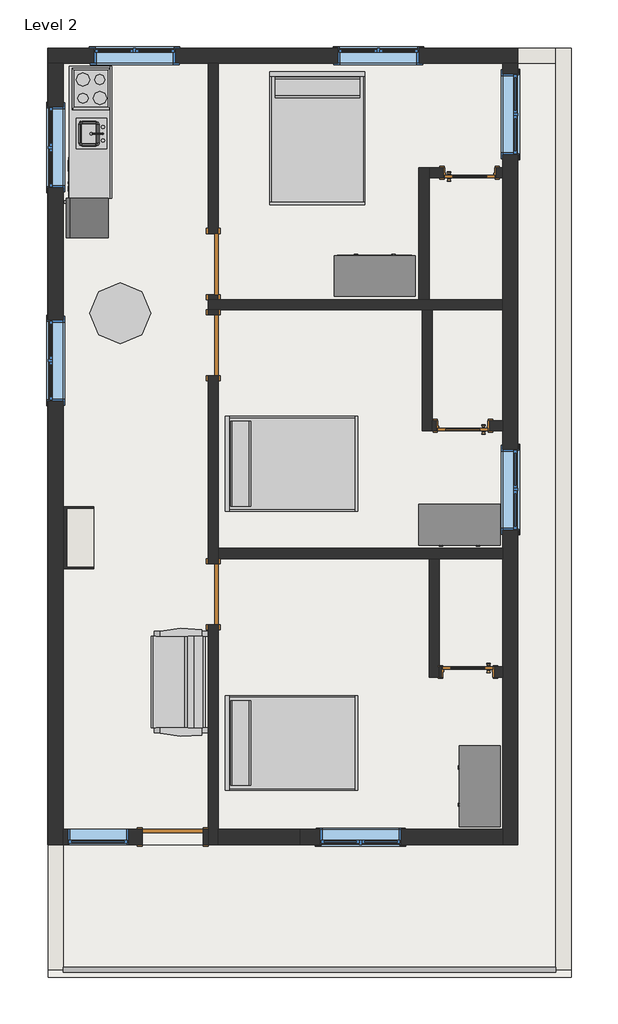
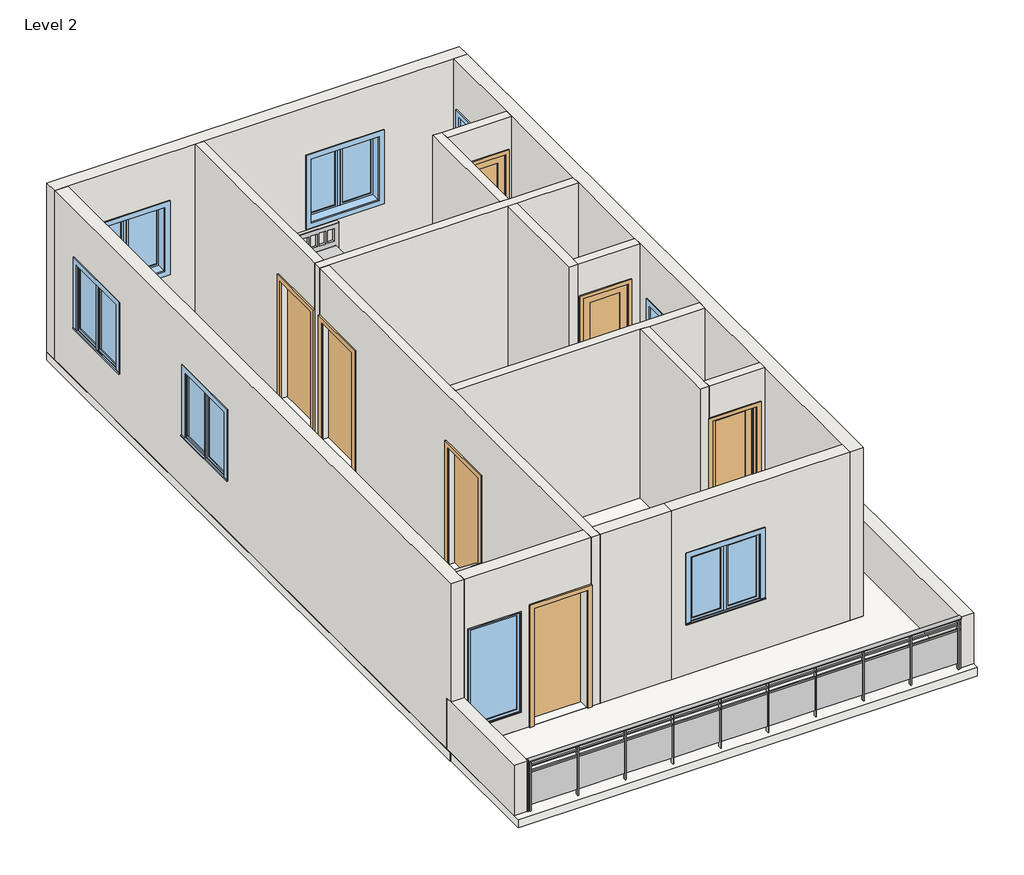
# One storey, incomplete: 20 walls, 9 furniture elements, 8 windows, 7 doors, 4 proxies, 2 slabs, 1 flow terminal, 1 railing.
# Revit data of these elements (continued)
# Element 50 (IfcWindow, "Casement Dbl with Trim : 48\" x 48\"") (continued)
#   Materials on its faces: "Sash", "Trim", "Glass"
# Element 51 (IfcWindow, "Casement Dbl with Trim : 48\" x 48\"")
#   Mark = "15"
#   Phase Created = New Construction
#   Materials on its faces: "Sash", "Trim", "Glass"
# Element 52 (IfcWindow, "Fixed : 36\" x 72\"")
#   Mark = "16"
#   Phase Created = New Construction
#   Materials on its faces: "Sash", "Glass"
# Materials
#   "Steel, Chrome Plated": class "Metal", colour RGB 17 17 17, transparency 0, Description = "Chromiuim plated steel", Cost = 0
#   "Steel, Polished": class "Metal", colour RGB 57 57 57, transparency 0, Description = "Polished steel", Cost = 0
#   "Steel, Paint Finish, Ivory, Glossy": class "Metal", colour RGB 247 247 239, transparency 0, Description = "Steel, paint finish, ivory, glossy", Cost = 0
#   "Plastic, Opaque Black": class "Plastic", colour RGB 0 0 0, transparency 0.7, Description = "Plastic, generic, opaque black", Cost = 0
#   "Cabinets": colour RGB 249 249 249, transparency 0
#   "Cabinets - Handles": class "Metal", colour RGB 57 57 57, transparency 0
#   "Cherry": class "Wood", colour RGB 226 177 128, transparency 0, Description = "Prunus Serotina", Cost = 0
#   "Aluminum": class "Metal", colour RGB 247 247 247, transparency 0, Description = "Aluminum 6061", Cost = 0
#   "Door - Panel": class "Wood", colour RGB 210 159 95, transparency 0
#   "Door - Frame": colour RGB 118 70 51, transparency 0
#   "Birch": class "Wood", colour RGB 224 178 126, transparency 0, Description = "Betula Alleghaniensis", Cost = 0
#   "Linen, White": class "Textile", colour RGB 247 247 239, transparency 0, Description = "Linen, white", Cost = 0
#   "Laminate - Ivory, Glossy": colour RGB 247 247 239, transparency 0
#   "Laminate, Ivory, Matte": class "Plastic", colour RGB 247 247 239, transparency 0, Description = "Plastic Laminate - Ivory, Matte", Cost = 0
#   "Linen, Beige": class "Textile", colour RGB 249 239 230, transparency 0, Description = "Linen, beige", Cost = 0
#   "Pine": class "Wood", colour RGB 223 192 134, transparency 0, Description = "Pinus Echinata", Cost = 0
#   "Laminate, Linen, Matte": class "Plastic", colour RGB 249 239 230, transparency 0, Description = "Plastic Laminate - Linen, Matte", Cost = 0
#   "FLOOR": class "Generic", colour RGB 144 129 110, transparency 0, Cost = 0
#   "EXT WALL": class "Generic", colour RGB 120 120 120, transparency 0, Cost = 0
#   "Glass": class "Glass", colour RGB 0 128 192, transparency 0.75, Description = "Soda Lime Glass", Cost = 0
#   "Sash": class "Wood", colour RGB 224 178 126, transparency 0
#   "Trim": class "Wood", colour RGB 224 178 126, transparency 0
#   "Counter Top": class "Wood", colour RGB 226 177 128, transparency 0
#   "Default Wall": colour RGB 128 128 128, transparency 0
